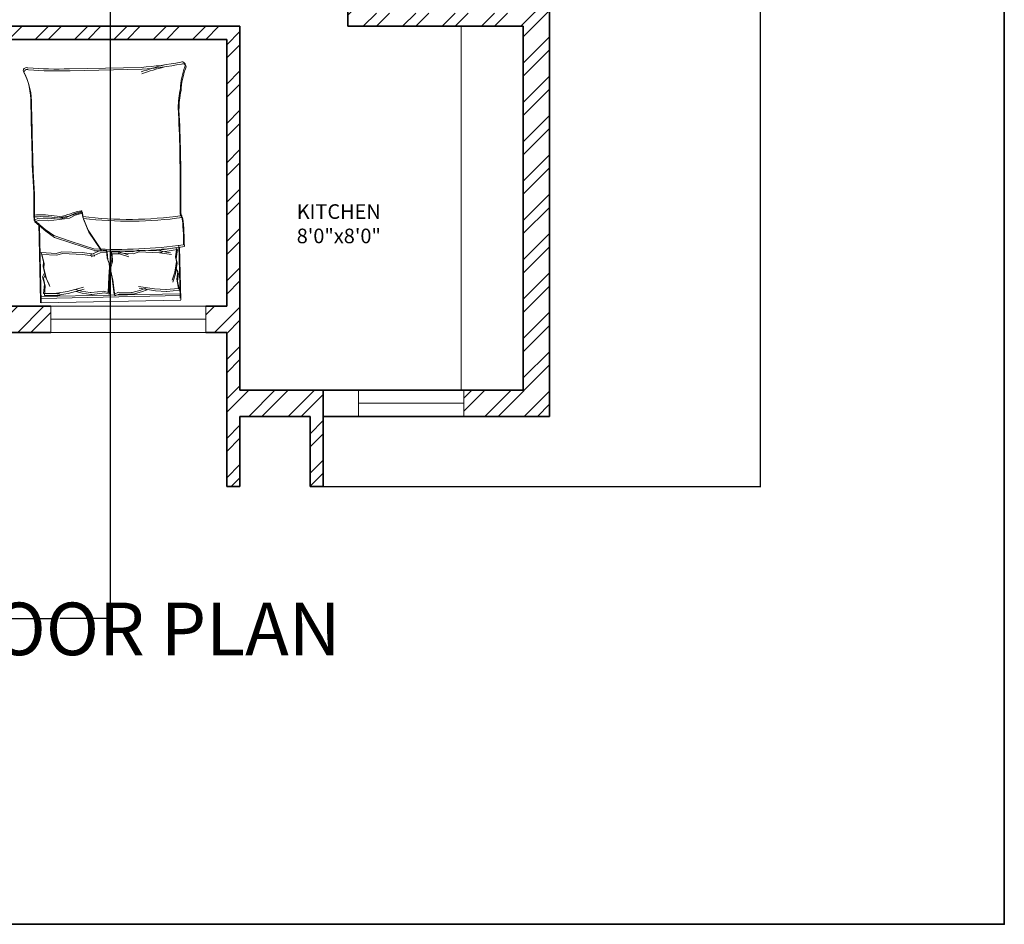
# Model space of a CAD drawing. Units: inches. Extents: x 1513 to 2170, y 1240 to 2288.
# Tile 3 of 10: x 1834 to 2170, y 1240 to 1549. Entities that reach past the tile are written whole.
import ezdxf

# ---------------------------------------------------------------- set-up
doc = ezdxf.new("R2010")
doc.units = ezdxf.units.IN
for name, color, linetype, lineweight in [('A-ANNO-DIMS', 2, 'Continuous', 18), ('A-ANNO-TTLB', 7, 'Continuous', 35), ('A-AREA-IDEN', 7, 'Continuous', 18), ('A-FLOR-FIXT', 9, 'Continuous', 18), ('A-FURN', 8, 'Continuous', 18), ('A-GLAZ', 4, 'Continuous', 18), ('A-WALL', 7, 'Continuous', 35), ('A-WALL-PATT', 252, 'Continuous', 13)]:
    doc.layers.add(name, color=color, linetype=linetype, lineweight=lineweight)
doc.styles.get("Standard").update_dxf_attribs({"font": 'arial.ttf'})
doc.dimstyles.get("Standard").update_dxf_attribs({"dimtxt": 0.18, "dimasz": 0.18, "dimexe": 0.18, "dimexo": 0.0625, "dimgap": 0.09, "dimtad": 0, "dimtih": 1, "dimtoh": 1, "dimdec": 4, "dimzin": 0, "dimdsep": 46, "dimtxsty": 'Standard', "dimcen": 0.09, "dimadec": 0, "dimazin": 0, "dimtfac": 1, "dimtdec": 4, "dimtofl": 0, "dimtmove": 0, "dimatfit": 3, "dimfxl": 1, "dimtolj": 1, "dimtzin": 0, "dimarcsym": 0})

# ---------------------------------------------------------------- blocks, each defined once
blk = doc.blocks.new('BED-DOUBLE')
for p, q in [((0, 51.27), (26.61, 51.27)), ((0, 51.27), (26.61, 51.27)), ((0.64, 51.49), (27.25, 51.49)), ((0.64, 51.49), (27.25, 51.49)), ((1.53, 3.48), (1.53, 51.27)), ((1.53, 3.48), (1.53, 51.27)), ((2.17, 3.7), (2.17, 51.49)), ((2.17, 3.7), (2.17, 51.49)), ((6.4, 49.96), (8.97, 50.56)), ((6.4, 49.96), (8.97, 50.56)), ((8.97, 50.56), (10.02, 50.04)), ((8.97, 50.56), (10.02, 50.04)), ((16.57, 50.7), (13.43, 49.92)), ((16.57, 50.7), (13.43, 49.92)), ((17.21, 50.93), (14.07, 50.15)), ((17.21, 50.93), (14.07, 50.15)), ((16.17, 45.57), (16.57, 50.7)), ((16.17, 45.57), (16.57, 50.7)), ((16.8, 45.8), (17.21, 50.93)), ((16.8, 45.8), (17.21, 50.93)), ((27.74, 52.87), (24.49, 49.16)), ((27.74, 52.87), (24.49, 49.16)), ((28.38, 53.1), (25.13, 49.39)), ((28.38, 53.1), (25.13, 49.39)), ((29.49, 52.95), (27.74, 52.87, 3.87)), ((29.49, 52.95), (27.74, 52.87, 3.87)), ((28.36, 51.33), (27.74, 52.87)), ((28.36, 51.33), (27.74, 52.87)), ((28.05, 48.23), (28.36, 51.33)), ((28.05, 48.23), (28.36, 51.33)), ((30.13, 53.18), (28.38, 53.1, 3.87)), ((30.13, 53.18), (28.38, 53.1, 3.87)), ((29, 51.56), (28.38, 53.1)), ((29, 51.56), (28.38, 53.1)), ((28.69, 48.46), (29, 51.56)), ((28.69, 48.46), (29, 51.56)), ((2.55, 50.11), (2.46, 44.71)), ((2.55, 50.11), (2.46, 44.71)), ((2.55, 50.11), (5.76, 49.73)), ((2.55, 50.11), (5.76, 49.73)), ((3.19, 50.34), (3.1, 44.94)), ((3.19, 50.34), (3.1, 44.94)), ((3.19, 50.34), (6.4, 49.96)), ((3.19, 50.34), (6.4, 49.96)), ((8.25, 49.31), (5.57, 48.13)), ((8.25, 49.31), (5.57, 48.13)), ((5.76, 49.73), (8.33, 50.33)), ((5.76, 49.73), (8.33, 50.33)), ((8.89, 49.54), (6.21, 48.36)), ((8.89, 49.54), (6.21, 48.36)), ((11.83, 50.11), (8.25, 49.31)), ((11.83, 50.11), (8.25, 49.31)), ((8.33, 50.33), (9.38, 49.82)), ((8.33, 50.33), (9.38, 49.82)), ((12.46, 50.34), (8.89, 49.54)), ((12.46, 50.34), (8.89, 49.54)), ((13.43, 49.92), (11.83, 50.11)), ((13.43, 49.92), (11.83, 50.11)), ((14.07, 50.15), (12.46, 50.34)), ((14.07, 50.15), (12.46, 50.34)), ((24.49, 49.16), (22.33, 46.22)), ((24.49, 49.16), (22.33, 46.22)), ((25.13, 49.39), (22.96, 46.45)), ((25.13, 49.39), (22.96, 46.45)), ((28.36, 44.36), (28.05, 48.23)), ((28.36, 44.36), (28.05, 48.23)), ((29, 44.59), (28.69, 48.46)), ((29, 44.59), (28.69, 48.46)), ((2.46, 44.71), (2.54, 45.71)), ((2.46, 44.71), (2.54, 45.71)), ((2.54, 45.71), (3.07, 41.92)), ((2.54, 45.71), (3.07, 41.92)), ((3.1, 44.94), (3.18, 45.94)), ((3.1, 44.94), (3.18, 45.94)), ((3.18, 45.94), (3.71, 42.14)), ((3.18, 45.94), (3.71, 42.14)), ((16.72, 43.61), (16.17, 45.57)), ((16.72, 43.61), (16.17, 45.57)), ((17.36, 43.84), (16.8, 45.8)), ((17.36, 43.84), (16.8, 45.8)), ((16.93, 36.83), (17.36, 43.84)), ((16.93, 36.83), (17.36, 43.84)), ((22.33, 46.22), (20.31, 40.65)), ((22.33, 46.22), (20.31, 40.65)), ((22.96, 46.45), (20.95, 40.87)), ((22.96, 46.45), (20.95, 40.87)), ((28.83, 40.96), (28.36, 44.36)), ((28.83, 40.95), (28.36, 44.36)), ((29.46, 41.18), (29, 44.59)), ((29.46, 41.18), (29, 44.59)), ((3.07, 41.92), (4.42, 36.5)), ((3.07, 41.92), (4.42, 36.5)), ((3.71, 42.14), (5.06, 36.72)), ((3.71, 42.14), (5.06, 36.72)), ((16.29, 36.6), (16.72, 43.61)), ((16.29, 36.6), (16.72, 43.61)), ((20.31, 40.65), (17.38, 32.31)), ((20.31, 40.65), (17.38, 32.31)), ((20.95, 40.87), (18.02, 32.54)), ((20.95, 40.87), (18.02, 32.54)), ((29.75, 38.94), (28.83, 40.96)), ((29.75, 38.94), (28.83, 40.95)), ((30.39, 39.17), (29.46, 41.18)), ((30.39, 39.17), (29.46, 41.18)), ((3.07, 37.14), (2.53, 34.21)), ((3.07, 37.14), (2.53, 34.21)), ((3.67, 39.2), (3.07, 37.14)), ((3.67, 39.2), (3.07, 37.14)), ((3.71, 37.36), (3.17, 34.43)), ((3.71, 37.36), (3.17, 34.43)), ((4.31, 39.43), (3.71, 37.36)), ((4.31, 39.43), (3.71, 37.36)), ((30.37, 36.46), (29.75, 38.94)), ((30.37, 36.46), (29.75, 38.94)), ((31.01, 36.69), (30.39, 39.17)), ((31.01, 36.69), (30.39, 39.17)), ((79.24, 15.06), (79.24, 39.68)), ((79.24, 15.06), (79.24, 39.68)), ((79.88, 15.29), (79.88, 39.91)), ((79.88, 15.29), (79.88, 39.91)), ((2.53, 34.21), (2.55, 33.88)), ((2.53, 34.21), (2.55, 33.88)), ((2.55, 33.88), (2.98, 29.46)), ((2.55, 33.88), (2.98, 29.46)), ((3.17, 34.43), (3.19, 34.11)), ((3.17, 34.43), (3.19, 34.11)), ((3.19, 34.11), (3.61, 29.69)), ((3.19, 34.11), (3.61, 29.68)), ((16.74, 30.75), (15.45, 33.82)), ((16.74, 30.75), (15.45, 33.82)), ((15.62, 32.57), (16.29, 36.6)), ((15.62, 32.57), (16.29, 36.6)), ((17.38, 30.98), (16.09, 34.05)), ((17.38, 30.98), (16.09, 34.05)), ((16.26, 32.79), (16.93, 36.83)), ((16.26, 32.79), (16.93, 36.83)), ((17.38, 30.26), (23.87, 34.45)), ((17.38, 30.26), (23.87, 34.45)), ((18.02, 30.49), (24.51, 34.68)), ((18.02, 30.49), (24.51, 34.68)), ((23.87, 34.45), (28.36, 36.15)), ((23.87, 34.45), (28.36, 36.15)), ((24.51, 34.68), (29, 36.38)), ((24.51, 34.68), (29, 36.38)), ((28.36, 36.15), (30.37, 36.46)), ((28.36, 36.15), (30.37, 36.46)), ((29, 36.38), (31.01, 36.69)), ((29, 36.38), (31.01, 36.69)), ((16.89, 28.3), (16.74, 30.75)), ((16.89, 28.3), (16.74, 30.75)), ((17.53, 28.53), (17.38, 30.98)), ((17.53, 28.53), (17.38, 30.98)), ((2.98, 29.46), (2.49, 27.98)), ((2.98, 29.46), (2.49, 27.98)), ((2.49, 27.98), (7.86, 27.73)), ((2.49, 27.98), (7.86, 27.73)), ((3.61, 29.69), (3.13, 28.21)), ((3.61, 29.68), (3.13, 28.21)), ((3.13, 28.21), (8.5, 27.96)), ((3.13, 28.21), (8.5, 27.96)), ((7.22, 26.56), (10.4, 27.14)), ((7.22, 26.56), (10.4, 27.14)), ((7.86, 27.73), (11.07, 27.36)), ((7.86, 27.73), (11.07, 27.36)), ((7.86, 26.79), (11.04, 27.37)), ((7.86, 26.79), (11.04, 27.37)), ((8.5, 27.96), (11.71, 27.58)), ((8.5, 27.96), (11.71, 27.58)), ((10.4, 27.14), (11.7, 27.14)), ((10.4, 27.14), (11.7, 27.14)), ((11.04, 27.37), (12.34, 27.37)), ((11.04, 27.37), (12.34, 27.37)), ((11.07, 27.36), (12.37, 27.44)), ((11.07, 27.36), (12.37, 27.44)), ((11.7, 27.14), (13.58, 26.56)), ((11.7, 27.14), (13.58, 26.56)), ((11.71, 27.58), (13.01, 27.67)), ((11.71, 27.58), (13.01, 27.67)), ((12.34, 27.37), (14.22, 26.79)), ((12.34, 27.37), (14.22, 26.79)), ((12.37, 27.44), (14.21, 28.13)), ((12.37, 27.44), (14.21, 28.13)), ((13.01, 27.67), (14.85, 28.36)), ((13.01, 27.67), (14.85, 28.36)), ((14.21, 28.13), (16.89, 28.3)), ((14.21, 28.13), (16.89, 28.3)), ((14.85, 28.36), (17.53, 28.53)), ((14.85, 28.36), (17.53, 28.53)), ((1.87, 25.98), (7.22, 26.56)), ((1.87, 25.98), (7.22, 26.56)), ((2.44, 24.54), (1.87, 25.98)), ((2.44, 24.54), (1.87, 25.98)), ((2.3, 20.09), (2.44, 24.54)), ((2.3, 20.09), (2.44, 24.54)), ((2.51, 26.21), (7.86, 26.79)), ((2.51, 26.21), (7.86, 26.79)), ((3.08, 24.77), (2.51, 26.21)), ((3.08, 24.77), (2.51, 26.21)), ((2.94, 20.32), (3.08, 24.77)), ((2.94, 20.32), (3.08, 24.77)), ((13.58, 26.56), (16.26, 26.56)), ((13.58, 26.56), (16.26, 26.56)), ((14.22, 26.79), (16.9, 26.79)), ((14.22, 26.79), (16.9, 26.79)), ((16.26, 24.1), (15.17, 20.96)), ((16.26, 24.1), (15.17, 20.96)), ((16.9, 24.33), (15.81, 21.19)), ((16.9, 24.33), (15.81, 21.19)), ((16.17, 19.39), (16.57, 24.52)), ((16.17, 19.38), (16.57, 24.52)), ((16.26, 26.56), (16.26, 24.1)), ((16.26, 26.56), (16.26, 24.1)), ((16.8, 19.61), (17.21, 24.75)), ((16.8, 19.61), (17.21, 24.74)), ((16.9, 26.79), (16.9, 24.33)), ((16.9, 26.79), (16.9, 24.33)), ((2.94, 20), (2.94, 20.32)), ((2.94, 20), (2.94, 20.32)), ((2.3, 19.77), (2.3, 20.09)), ((2.3, 19.77), (2.3, 20.09)), ((3.02, 16.88), (2.3, 19.77)), ((3.02, 16.88), (2.3, 19.77)), ((3.66, 17.11), (2.94, 20)), ((3.66, 17.11), (2.94, 20)), ((3.75, 14.86), (3.02, 16.88)), ((3.75, 14.86), (3.02, 16.88)), ((3.31, 12.11), (4.32, 17.6)), ((3.31, 12.11), (4.32, 17.6)), ((4.39, 15.08), (3.66, 17.11)), ((4.39, 15.08), (3.66, 17.11)), ((3.95, 12.34), (4.96, 17.83)), ((3.95, 12.34), (4.96, 17.83)), ((16.72, 17.42), (16.17, 19.39)), ((16.72, 17.42), (16.17, 19.38)), ((16.29, 10.41), (16.72, 17.42)), ((16.29, 10.41), (16.72, 17.42)), ((17.36, 17.65), (16.8, 19.61)), ((17.36, 17.65), (16.8, 19.61)), ((16.93, 10.64), (17.36, 17.65)), ((16.93, 10.64), (17.36, 17.65)), ((3.02, 8.29), (3.31, 12.11)), ((3.02, 8.29), (3.31, 12.11)), ((3.66, 8.51), (3.95, 12.34)), ((3.66, 8.51), (3.95, 12.34)), ((15.62, 6.38), (16.29, 10.41)), ((15.62, 6.38), (16.29, 10.41)), ((16.26, 6.61), (16.93, 10.64)), ((16.26, 6.61), (16.93, 10.64)), ((16.29, 10.41), (16.61, 9.28)), ((16.29, 10.41), (16.61, 9.28)), ((16.93, 10.64), (17.25, 9.51)), ((16.93, 10.64), (17.25, 9.51)), ((3.01, 8.18), (3.02, 8.29)), ((3.01, 8.18), (3.02, 8.29)), ((3.33, 3.9), (3.01, 8.18)), ((3.33, 3.9), (3.01, 8.18)), ((3.64, 8.41), (3.66, 8.51)), ((3.64, 8.41), (3.66, 8.51)), ((3.97, 4.13), (3.64, 8.41)), ((3.97, 4.13), (3.64, 8.41)), ((16.61, 9.28), (17.34, 4.18)), ((16.61, 9.28), (17.34, 4.18)), ((17.25, 9.51), (17.98, 4.41)), ((17.25, 9.51), (17.98, 4.41)), ((18.11, 3.48), (0, 3.48)), ((18.11, 3.48), (0, 3.48)), ((18.75, 3.7), (0.64, 3.7)), ((18.75, 3.7), (0.64, 3.7)), ((3.31, 3.9), (6.49, 4.47)), ((3.31, 3.9), (6.49, 4.47)), ((3.95, 4.12), (7.13, 4.7)), ((3.95, 4.12), (7.13, 4.7)), ((8.95, 5.05), (6.2, 6.06)), ((8.95, 5.05), (6.2, 6.06)), ((6.49, 4.47), (9.1, 4.04)), ((6.49, 4.47), (9.1, 4.04)), ((9.59, 5.28), (6.84, 6.29)), ((9.59, 5.28), (6.84, 6.29)), ((7.13, 4.7), (9.74, 4.27)), ((7.13, 4.7), (9.74, 4.27)), ((12.57, 4.47), (8.95, 5.05)), ((12.57, 4.47), (8.95, 5.05)), ((9.1, 4.04), (10.11, 4.62)), ((9.1, 4.04), (10.11, 4.62)), ((13.21, 4.7), (9.59, 5.28)), ((13.21, 4.7), (9.59, 5.28)), ((9.74, 4.27), (10.75, 4.85)), ((9.74, 4.27), (10.75, 4.85)), ((14.16, 4.76), (12.57, 4.47)), ((14.16, 4.76), (12.57, 4.47)), ((14.8, 4.99), (13.21, 4.7)), ((14.8, 4.99), (13.21, 4.7)), ((17.34, 4.18), (14.16, 4.76)), ((17.34, 4.18), (14.16, 4.76)), ((17.98, 4.41), (14.8, 4.99)), ((17.98, 4.41), (14.8, 4.99))]:
    blk.add_line(p, q)
for centre, radius, start, end in [((68.66, 76.16), 23.07, 267.4714, 296.4681), ((68.66, 76.16), 23.07, 267.4714, 296.4681), ((69.3, 76.39), 23.07, 267.4714, 296.4681), ((69.3, 76.39), 23.07, 267.4714, 296.4681), ((78.87, 54.41), 1.1, 332.6588, 86.02), ((78.87, 54.41), 1.1, 332.6588, 86.02), ((79.51, 54.64), 1.1, 332.6588, 86.02), ((79.51, 54.64), 1.1, 332.6588, 86.02), ((212.91, 41.38), 133.04, 174.4998, 180.6351), ((212.91, 41.38), 133.04, 174.4998, 180.6351), ((-6.66, 51.33), 36.18, 349.8763, 2.5657), ((-6.66, 51.33), 36.18, 349.8763, 2.5657), ((36.31, 182.27), 129.5, 266.9791, 273.8365), ((36.31, 182.27), 129.5, 266.9791, 273.8365), ((-6.02, 51.56), 36.18, 349.8763, 2.5657), ((-6.02, 51.56), 36.18, 349.8763, 2.5657), ((36.95, 182.5), 129.5, 266.9791, 273.8365), ((36.95, 182.5), 129.5, 266.9791, 273.8365), ((67.82, -4508.74), 4561.86, 90.00217, 90.28689), ((67.82, -4508.74), 4561.86, 90.00217, 90.28689), ((68.46, -4508.51), 4561.86, 90.00217, 90.28689), ((68.46, -4508.51), 4561.86, 90.00217, 90.28689), ((212.27, 41.15), 133.04, 174.4998, 180.6351), ((212.27, 41.15), 133.04, 174.4998, 180.6351), ((35.06, 43.74), 6.22, 168.6608, 203.7384), ((35.06, 43.74), 6.22, 168.6608, 203.7384), ((35.7, 43.97), 6.22, 168.6608, 203.7384), ((35.7, 43.97), 6.22, 168.6608, 203.7384), ((1.48, 31.15), 29.65, 10.6617, 19.8806), ((1.48, 31.15), 29.65, 10.6617, 19.8806), ((2.12, 31.38), 29.65, 10.6617, 19.8806), ((2.12, 31.38), 29.65, 10.6617, 19.8806), ((156.31, 17.76), 129.02, 171.7845, 186.9006), ((156.31, 17.76), 129.02, 171.7845, 186.9006), ((156.95, 17.99), 129.02, 171.7845, 186.9006), ((156.95, 17.98), 129.02, 171.7845, 186.9006), ((30.44, 36.64), 0.185, 250.2464, 1.1377), ((30.44, 36.64), 0.185, 250.2464, 1.1377), ((31.08, 36.87), 0.185, 250.2464, 1.1377), ((31.08, 36.87), 0.185, 250.2464, 1.1377), ((182.05, 21.36), 164.97, 176.0865, 186.7821), ((182.05, 21.36), 164.97, 176.0865, 186.7821), ((182.69, 21.59), 164.97, 176.0865, 186.7821), ((182.69, 21.59), 164.97, 176.0865, 186.7821), ((-23.72, -17.22), 106.46, 13.3832, 17.7053), ((-23.72, -17.22), 106.46, 13.3832, 17.7053), ((-23.08, -16.99), 106.46, 13.3832, 17.7053), ((-23.08, -16.99), 106.46, 13.3832, 17.7053), ((200.83, 21.43), 121.76, 182.9958, 189.4091), ((200.83, 21.43), 121.76, 182.9958, 189.4091), ((201.47, 21.66), 121.76, 182.9958, 189.4091), ((201.47, 21.66), 121.76, 182.9958, 189.4091), ((20.09, 85.16), 83.31, 268.7218, 275.604), ((20.09, 85.16), 83.31, 268.7218, 275.604), ((20.73, 85.39), 83.31, 268.7218, 275.604), ((20.73, 85.39), 83.31, 268.7218, 275.604), ((31.17, -167.31), 170.11, 88.4762, 91.0082), ((31.17, -167.31), 170.11, 88.4762, 91.0082), ((31.81, -167.08), 170.11, 88.4762, 91.0082), ((31.81, -167.08), 170.11, 88.4762, 91.0082), ((50.61, 484.82), 482.31, 268.2277, 271.7185), ((50.61, 484.82), 482.31, 268.2277, 271.7185), ((51.25, 485.05), 482.31, 268.2277, 271.7185), ((51.25, 485.05), 482.31, 268.2277, 271.7185), ((64.51, -26.9), 29.63, 76.0648, 88.9113), ((64.51, -26.9), 29.63, 76.0648, 88.9113), ((65.15, -26.67), 29.63, 76.0648, 88.9113), ((65.15, -26.67), 29.63, 76.0648, 88.9113), ((70.27, -21.66), 23.56, 67.9751, 86.652), ((70.27, -21.66), 23.56, 67.9751, 86.652), ((70.91, -21.43), 23.56, 67.9751, 86.652), ((70.91, -21.43), 23.56, 67.9751, 86.652), ((79.71, 1.09), 1.09, 236.1736, 23.4781), ((79.71, 1.09), 1.09, 236.1736, 23.4781), ((80.35, 1.32), 1.09, 236.1736, 23.4781), ((80.35, 1.32), 1.09, 236.1736, 23.4781)]:
    blk.add_arc(centre, radius, start, end)
blk = doc.blocks.new('*D26')
at = {"layer": 'A-ANNO-DIMS', "color": 0, "lineweight": -2, "transparency": 16777216}
for p, q in [((2014.91, 2214.48), (2087.18, 2214.48)), ((2087, 2214.3), (2087, 1802.16)), ((2087, 1389.66), (2087, 1801.8)), ((1937.43, 1389.48), (2087.18, 1389.48))]:
    blk.add_line(p, q, dxfattribs=at)
at = {"layer": 'A-ANNO-DIMS', "color": 0, "transparency": 16777216}
for points in [[(2086.97, 2214.3), (2087.03, 2214.3), (2087, 2214.48)], [(2086.97, 1389.66), (2087.03, 1389.66), (2087, 1389.48)]]:
    blk.add_solid(points, dxfattribs=at)
at = {"layer": 'Defpoints', "color": 0, "transparency": 16777216}
for p in [(2014.85, 2214.48), (2087, 2214.48), (1937.37, 1389.48)]:
    blk.add_point(p, dxfattribs=at)
at = {"layer": 'A-ANNO-DIMS', "color": 0, "transparency": 16777216, "insert": (2087, 1801.98), "char_height": 0.18, "attachment_point": 5}
blk.add_mtext('\\A1;825', dxfattribs=at)
blk = doc.blocks.new('*D36')
at = {"layer": 'A-ANNO-DIMS', "color": 0, "lineweight": -2, "transparency": 16777216}
for p, q in [((1829.49, 1887.42), (1829.49, 1344.15)), ((1864.51, 1887.42), (1864.51, 1344.15)), ((1829.67, 1344.33), (1846.61, 1344.33)), ((1864.33, 1344.33), (1847.39, 1344.33))]:
    blk.add_line(p, q, dxfattribs=at)
at = {"layer": 'A-ANNO-DIMS', "color": 0, "transparency": 16777216}
for points in [[(1829.67, 1344.36), (1829.67, 1344.3), (1829.49, 1344.33)], [(1864.33, 1344.36), (1864.33, 1344.3), (1864.51, 1344.33)]]:
    blk.add_solid(points, dxfattribs=at)
at = {"layer": 'Defpoints', "color": 0, "transparency": 16777216}
for p in [(1829.49, 1887.48), (1864.51, 1887.48), (1864.51, 1344.33)]:
    blk.add_point(p, dxfattribs=at)
at = {"layer": 'A-ANNO-DIMS', "color": 0, "transparency": 16777216, "insert": (1847, 1344.33), "char_height": 0.18, "attachment_point": 5}
blk.add_mtext('\\A1;35.02', dxfattribs=at)

msp = doc.modelspace()

# ---------------------------------------------------------------- hatches: boundary and pattern name
at = {"layer": 'A-WALL-PATT'}
h = msp.add_hatch(dxfattribs=at)
h.set_pattern_fill('ANSI32', color=256)
h.paths.add_polyline_path([(2041.852, 1719.48), (2014.852, 1719.48), (2014.852, 1734.444), (2005.852, 1734.444), (2005.852, 1710.48), (2032.852, 1710.48), (2032.852, 1663.98), (1976.619, 1663.98), (1976.619, 1659.48), (2005.852, 1659.48), (2005.852, 1626.27), (2014.852, 1626.27), (2014.852, 1659.48), (2041.852, 1659.48)])
h.paths.add_polyline_path([(1954.521, 1663.98), (1875.357, 1663.98), (1875.357, 1659.48), (1945.852, 1659.48), (1945.852, 1546.98), (1950.352, 1546.98), (2005.852, 1546.98), (2005.852, 1422.48), (1985.47, 1422.48), (1985.47, 1413.48), (2014.852, 1413.48), (2014.852, 1602.27), (2005.852, 1602.27), (2005.852, 1551.48), (1950.352, 1551.48), (1950.352, 1659.48), (1954.521, 1659.48)])
h.paths.add_polyline_path([(1949.47, 1422.48), (1937.366, 1422.48), (1937.366, 1413.48), (1949.47, 1413.48)], flags=0)
h.paths.add_polyline_path([(1937.366, 1422.48), (1908.866, 1422.48), (1908.866, 1546.98), (1805.486, 1546.98), (1805.486, 1542.48), (1904.366, 1542.48), (1904.366, 1451.2), (1897.222, 1451.2), (1897.222, 1442.2), (1904.366, 1442.2), (1904.366, 1422.48), (1904.366, 1413.48), (1904.366, 1389.48), (1908.866, 1389.48), (1908.866, 1413.48), (1932.866, 1413.48), (1932.866, 1389.48), (1937.366, 1389.48)])
h.paths.add_polyline_path([(1830.254, 1442.2), (1844.144, 1442.2), (1844.144, 1451.2), (1830.254, 1451.2), (1821.254, 1451.2), (1821.254, 1422.48), (1766.366, 1422.48), (1766.366, 1542.48), (1770.265, 1542.48), (1770.265, 1546.98), (1758.774, 1546.98), (1758.774, 1544.73), (1758.774, 1542.48), (1761.866, 1542.48), (1761.866, 1389.48), (1779.454, 1389.48), (1779.454, 1398.48), (1770.866, 1398.48), (1770.866, 1413.48), (1830.254, 1413.48)])
h.paths.add_polyline_path([(1686.156, 1451.2), (1677.156, 1451.2), (1677.156, 1422.48), (1623.866, 1422.48), (1623.866, 1460.073), (1614.866, 1460.073), (1614.866, 1413.48), (1686.156, 1413.48)])
h.paths.add_polyline_path([(1761.866, 1422.48), (1686.156, 1422.48), (1686.156, 1413.48), (1761.866, 1413.48)])
h.paths.add_polyline_path([(1623.866, 1542.48), (1688.266, 1542.48), (1688.266, 1544.73), (1688.266, 1546.98), (1623.866, 1546.98), (1623.866, 1560.442), (1614.866, 1560.442), (1614.866, 1520.073), (1619.366, 1520.073), (1623.866, 1520.073)])
h.paths.add_polyline_path([(1623.866, 1600.98), (1715.366, 1600.98), (1715.366, 1546.98), (1711.055, 1546.98), (1711.055, 1542.48), (1719.866, 1542.48), (1726.867, 1542.48), (1726.867, 1544.73), (1726.867, 1546.98), (1719.866, 1546.98), (1719.866, 1600.98), (1719.866, 1608.301), (1717.616, 1608.301), (1715.366, 1608.301), (1715.366, 1605.48), (1623.866, 1605.48), (1623.866, 1620.254), (1614.866, 1620.254), (1614.866, 1584.442), (1623.866, 1584.442)])
h.paths.add_polyline_path([(1623.866, 1659.48), (1715.366, 1659.48), (1715.366, 1629.2), (1719.866, 1629.2), (1719.866, 1659.48), (1767.866, 1659.48), (1767.866, 1629.2), (1772.366, 1629.2), (1772.366, 1663.98), (1578.866, 1663.98), (1578.866, 1661.73), (1578.866, 1659.48), (1578.866, 1635.48), (1583.366, 1635.48), (1583.366, 1654.98), (1614.866, 1654.98), (1614.866, 1644.254), (1619.366, 1644.254), (1623.866, 1644.254)])
h.paths.add_polyline_path([(1788.587, 1798.98), (1788.587, 1803.48), (1623.866, 1803.48), (1623.866, 1887.48), (1829.49, 1887.48), (1829.49, 1891.98), (1829.49, 1896.48), (1748.366, 1896.48), (1743.866, 1896.48), (1623.866, 1896.48), (1623.866, 1904.333), (1619.366, 1904.333), (1614.866, 1904.333), (1614.866, 1896.48), (1578.866, 1896.48), (1578.866, 1887.48), (1614.866, 1887.48), (1614.866, 1803.48), (1578.866, 1803.48), (1578.866, 1794.48), (1626.866, 1794.48), (1788.587, 1794.48)])
h.paths.add_polyline_path([(1635.866, 1794.48), (1626.866, 1794.48), (1626.866, 1763.627), (1631.366, 1763.627), (1635.866, 1763.627)])
h.paths.add_polyline_path([(1635.866, 1703.627), (1626.866, 1703.627), (1626.866, 1663.98), (1635.866, 1663.98)])
h.paths.add_polyline_path([(1587.866, 2016.48), (1614.866, 2016.48), (1623.866, 2016.48), (1707.767, 2016.48), (1707.767, 2018.73), (1707.767, 2020.98), (1706.366, 2020.98), (1706.366, 2025.944), (1701.866, 2025.944), (1701.866, 2020.98), (1623.866, 2020.98), (1623.866, 2045.903), (1614.866, 2045.903), (1614.866, 2025.48), (1583.366, 2025.48), (1583.366, 2040.48), (1578.866, 2040.48), (1578.866, 2016.48), (1578.866, 1956.48), (1614.866, 1956.48), (1614.866, 1946.333), (1623.866, 1946.333), (1623.866, 1965.48), (1587.866, 1965.48)])
h.paths.add_polyline_path([(1748.366, 2016.48), (1748.366, 2025.48), (1743.866, 2025.48), (1739.366, 2025.48), (1739.366, 2020.98), (1738.09, 2020.98), (1738.09, 2016.48), (1743.866, 2016.48), (1743.866, 1896.48), (1748.366, 1896.48)])
h.paths.add_polyline_path([(1746.736, 2085.48), (1623.866, 2085.48), (1623.866, 2205.48), (1657.136, 2205.48), (1657.136, 2214.48), (1614.866, 2214.48), (1614.866, 2069.903), (1623.866, 2069.903), (1623.866, 2080.98), (1683.866, 2080.98), (1701.866, 2080.98), (1701.866, 2046.743), (1706.366, 2046.743), (1706.366, 2080.98), (1746.736, 2080.98)])

# ---------------------------------------------------------------- linework, layer by layer
at = {"layer": 'A-ANNO-TTLB'}
msp.add_lwpolyline([(1513.071, 2287.731), (2170.435, 2287.731), (2170.435, 1239.669), (1513.071, 1239.669)], close=True, dxfattribs=at)
at = {"layer": 'A-FLOR-FIXT'}
msp.add_line((1984.568, 1546.98), (1984.568, 1422.48), dxfattribs=at)
at = {"layer": 'A-FURN'}
for p, q in [((1840.636, 1452.299), (1840.623, 1452.938)), ((1840.864, 1452.304), (1888.644, 1453.307))]:
    msp.add_line(p, q, dxfattribs=at)
at = {"layer": 'A-GLAZ'}
for p, q in [((1844.144, 1442.2), (1844.144, 1451.2)), ((1844.144, 1451.2), (1897.222, 1451.2)), ((1897.222, 1451.2), (1897.222, 1442.2)), ((1897.222, 1446.7), (1844.144, 1446.7)), ((1897.222, 1442.2), (1897.222, 1446.7)), ((1844.144, 1442.2), (1897.222, 1442.2)), ((1949.47, 1417.98), (1949.47, 1422.48)), ((1949.47, 1422.48), (1949.47, 1413.48)), ((1985.47, 1422.48), (1985.47, 1413.48)), ((1985.47, 1417.98), (1949.47, 1417.98)), ((1985.47, 1413.48), (1985.47, 1417.98))]:
    msp.add_line(p, q, dxfattribs=at)
at = {"layer": 'A-WALL'}
for p, q in [((1945.852, 1546.98), (1945.852, 1659.48)), ((2014.852, 1413.48), (2014.852, 1659.48)), ((1805.486, 1546.98), (1908.866, 1546.98)), ((1904.366, 1546.98), (1908.866, 1546.98)), ((1908.866, 1546.98), (1908.866, 1422.48)), ((1908.866, 1546.98), (1908.866, 1542.48)), ((1950.352, 1546.98), (1945.852, 1546.98)), ((2005.852, 1546.98), (1950.352, 1546.98)), ((2005.852, 1546.98), (2005.852, 1422.48)), ((1904.366, 1542.48), (1803.73, 1542.48)), ((1904.366, 1451.2), (1904.366, 1542.48)), ((1844.144, 1451.2), (1830.254, 1451.2)), ((1897.222, 1451.2), (1904.366, 1451.2)), ((1830.254, 1442.2), (1844.144, 1442.2)), ((1897.222, 1442.2), (1904.366, 1442.2)), ((1904.366, 1422.48), (1904.366, 1442.2)), ((1904.366, 1422.48), (1904.366, 1413.48)), ((1908.866, 1422.48), (2005.852, 1422.48)), ((1937.366, 1389.48), (1937.366, 1422.48)), ((1904.366, 1413.48), (1904.366, 1389.48)), ((1908.866, 1389.48), (1908.866, 1413.48)), ((1908.866, 1413.48), (1932.866, 1413.48)), ((1908.866, 1413.48), (1932.866, 1413.48)), ((1932.866, 1413.48), (1932.866, 1389.48)), ((1937.366, 1413.48), (2014.852, 1413.48)), ((1904.366, 1389.48), (1908.866, 1389.48)), ((1932.866, 1389.48), (1937.366, 1389.48))]:
    msp.add_line(p, q, dxfattribs=at)

# ---------------------------------------------------------------- block references
at = {"layer": 'A-FURN', "rotation": 91.2026117603728}
msp.add_blockref('BED-DOUBLE', (1892.119, 1453.383), dxfattribs=at)

# ---------------------------------------------------------------- texts
at = {"layer": 'A-ANNO-TTLB', "insert": (1726.168, 1349.749), "char_height": 18, "attachment_point": 1}
msp.add_mtext_dynamic_manual_height_columns('FIRST FLOOR PLAN', width=444.32669, gutter_width=12.5, heights=[0], dxfattribs=at)
at = {"layer": 'A-AREA-IDEN', "insert": (1928.32, 1486.069), "char_height": 5, "attachment_point": 1}
msp.add_mtext_dynamic_manual_height_columns('KITCHEN\\P8\'0"x8\'0"', width=289.28651, gutter_width=12.5, heights=[0], dxfattribs=at)

# ---------------------------------------------------------------- dimensions: what is measured, and where the dimension line sits
at = {"layer": 'A-ANNO-DIMS'}
dim = msp.add_linear_dim(base=(2087.002, 2214.48), p1=(1937.366, 1389.48), p2=(2014.852, 2214.48), angle=90, dimstyle='Standard', override={"dimdec": 0, "dimlfac": 1, "dimrnd": 0, "dimzin": 0, "dimdsep": 46, "dimlunit": 2}, dxfattribs=at)
dim.commit()
dim.dimension.update_dxf_attribs({"geometry": '*D26', "text_midpoint": (2087.002, 1801.98)})
dim = msp.add_linear_dim(base=(1864.508, 1344.33), p1=(1829.49, 1887.48), p2=(1864.508, 1887.48), dimstyle='Standard', override={"dimdec": 2, "dimlfac": 1, "dimrnd": 0, "dimzin": 0, "dimdsep": 46, "dimlunit": 2}, dxfattribs=at)
dim.commit()
dim.dimension.update_dxf_attribs({"geometry": '*D36', "text_midpoint": (1846.999, 1344.33)})

doc.saveas('drawing.dxf')
